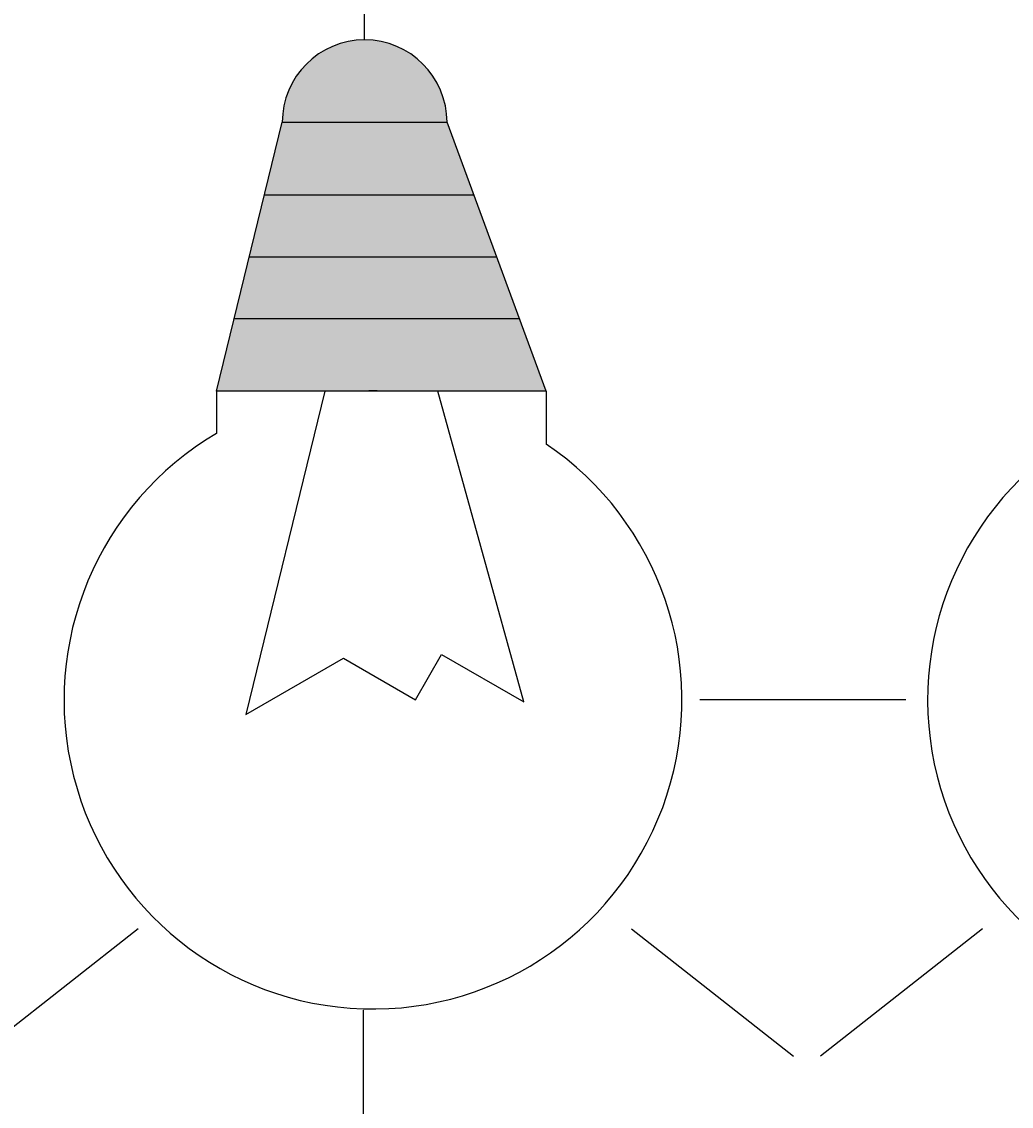
# Model space of a CAD drawing. Units: millimetres. Extents: x -8 to 285, y 5 to 221.
# Tile 26 of 30: x 172 to 221, y 132 to 185. Entities that reach past the tile are written whole.
import ezdxf

# ---------------------------------------------------------------- set-up
doc = ezdxf.new("R2010")
doc.units = ezdxf.units.MM
for name, color, linetype, lineweight in [('A-ANNO-DIMS', 2, 'Continuous', 18), ('E-EQPM-PATT', 252, 'Continuous', 13), ('E-LITE-FIXT', 7, 'Continuous', 25)]:
    doc.layers.add(name, color=color, linetype=linetype, lineweight=lineweight)
doc.layers.add('E-POWR-AC-LINE', color=30, linetype='Continuous', lineweight=25, true_color=0xf26722)
doc.styles.get("Standard").update_dxf_attribs({"font": 'arial.ttf'})
doc.dimstyles.get("Standard").update_dxf_attribs({"dimtxt": 0.18, "dimasz": 0.18, "dimexe": 0.18, "dimexo": 0.0625, "dimgap": 0.09, "dimtad": 0, "dimtih": 1, "dimtoh": 1, "dimdec": 4, "dimzin": 0, "dimdsep": 46, "dimtxsty": 'Standard', "dimcen": 0.09, "dimadec": 0, "dimazin": 0, "dimtfac": 1, "dimtdec": 4, "dimtofl": 0, "dimtmove": 0, "dimatfit": 3, "dimfxl": 1, "dimtolj": 1, "dimtzin": 0, "dimarcsym": 0})

# ---------------------------------------------------------------- blocks, each defined once
blk = doc.blocks.new('LAMP-INCANDESCENT')
for p, q in [((7.407, 29.994), (10.595, 43.039)), ((23.407, 29.994), (18.595, 43.039)), ((9.734, 39.517), (19.894, 39.517)), ((9.001, 36.517), (21.001, 36.517)), ((8.268, 33.517), (22.107, 33.517)), ((7.407, 29.994), (7.407, 27.935)), ((12.666, 29.994), (8.834, 14.293)), ((22.321, 14.903), (18.146, 29.994)), ((23.407, 29.994), (23.407, 27.423)), ((8.834, 14.293), (13.574, 17.029)), ((13.574, 17.029), (17.067, 15.012)), ((17.067, 15.012), (18.333, 17.205)), ((18.333, 17.205), (22.321, 14.903))]:
    blk.add_line(p, q)
for points in [[(10.595, 43.039), (18.595, 43.039)], [(23.407, 29.994), (7.407, 29.994)]]:
    blk.add_lwpolyline(points)
for centre, radius, start, end in [((14.595, 43.039), 4, 0, 180), ((15.001, 15), 15, 88.4488, 91.5512), ((15.001, 15), 15, 120.4152, 55.9163)]:
    blk.add_arc(centre, radius, start, end)
blk = doc.blocks.new('*D9')
at = {"layer": 'A-ANNO-DIMS', "color": 0, "lineweight": -2, "transparency": 16777216}
for p, q in [((6.672, 133.79), (6.672, 220.737)), ((270.919, 206.519), (270.919, 220.737)), ((6.852, 220.557), (138.33, 220.557)), ((270.739, 220.557), (139.262, 220.557))]:
    blk.add_line(p, q, dxfattribs=at)
at = {"layer": 'A-ANNO-DIMS', "color": 0, "transparency": 16777216}
for points in [[(6.852, 220.587), (6.852, 220.527), (6.672, 220.557)], [(270.739, 220.587), (270.739, 220.527), (270.919, 220.557)]]:
    blk.add_solid(points, dxfattribs=at)
at = {"layer": 'Defpoints', "color": 0, "transparency": 16777216}
for p in [(270.919, 220.557), (270.919, 206.457), (6.672, 133.727)]:
    blk.add_point(p, dxfattribs=at)
at = {"layer": 'A-ANNO-DIMS', "color": 0, "transparency": 16777216, "insert": (138.796, 220.557), "char_height": 0.18, "attachment_point": 5}
blk.add_mtext('\\A1;264.25', dxfattribs=at)
blk = doc.blocks.new('*D13')
at = {"layer": 'A-ANNO-DIMS', "color": 0, "lineweight": -2, "transparency": 16777216}
for p, q in [((145.21, 137.013), (145.21, 5.222)), ((189.039, 137.013), (189.039, 5.222)), ((145.39, 5.402), (166.727, 5.402)), ((188.859, 5.402), (167.522, 5.402))]:
    blk.add_line(p, q, dxfattribs=at)
at = {"layer": 'A-ANNO-DIMS', "color": 0, "transparency": 16777216}
for points in [[(145.39, 5.432), (145.39, 5.372), (145.21, 5.402)], [(188.859, 5.432), (188.859, 5.372), (189.039, 5.402)]]:
    blk.add_solid(points, dxfattribs=at)
at = {"layer": 'Defpoints', "color": 0, "transparency": 16777216}
for p in [(145.21, 137.075), (189.039, 137.075), (189.039, 5.402)]:
    blk.add_point(p, dxfattribs=at)
at = {"layer": 'A-ANNO-DIMS', "color": 0, "transparency": 16777216, "insert": (167.124, 5.402), "char_height": 0.18, "attachment_point": 5}
blk.add_mtext('\\A1;43.83', dxfattribs=at)
blk = doc.blocks.new('*D14')
at = {"layer": 'A-ANNO-DIMS', "color": 0, "lineweight": -2, "transparency": 16777216}
for p, q in [((189.039, 137.013), (189.039, 5.222)), ((230.967, 137.013), (230.967, 5.222)), ((189.219, 5.402), (209.606, 5.402)), ((230.787, 5.402), (210.4, 5.402))]:
    blk.add_line(p, q, dxfattribs=at)
at = {"layer": 'A-ANNO-DIMS', "color": 0, "transparency": 16777216}
for points in [[(189.219, 5.432), (189.219, 5.372), (189.039, 5.402)], [(230.787, 5.432), (230.787, 5.372), (230.967, 5.402)]]:
    blk.add_solid(points, dxfattribs=at)
at = {"layer": 'Defpoints', "color": 0, "transparency": 16777216}
for p in [(189.039, 137.075), (230.967, 137.075), (230.967, 5.402)]:
    blk.add_point(p, dxfattribs=at)
at = {"layer": 'A-ANNO-DIMS', "color": 0, "transparency": 16777216, "insert": (210.003, 5.402), "char_height": 0.18, "attachment_point": 5}
blk.add_mtext('\\A1;41.93', dxfattribs=at)

msp = doc.modelspace()

# ---------------------------------------------------------------- hatches: boundary and pattern name
at = {"layer": 'E-EQPM-PATT'}
h = msp.add_hatch(color=256, dxfattribs=at)
h.set_gradient(color1=(0, 0, 255), color2=(34, 52, 110), tint=1)
h.paths.add_polyline_path([(141.2836, 180.1071), (149.2836, 180.1071, 1)])
h.paths.add_polyline_path([(149.2836, 180.1071), (141.2836, 180.1071), (140.4228, 176.5846), (150.583, 176.5846)])
h.paths.add_polyline_path([(150.583, 176.5846), (140.4228, 176.5846), (139.6897, 173.5846), (151.6897, 173.5846)])
h.paths.add_polyline_path([(151.6897, 173.5846), (139.6897, 173.5846), (138.9565, 170.5846), (152.7963, 170.5846)])
h.paths.add_polyline_path([(152.7963, 170.5846), (138.9565, 170.5846), (138.0957, 167.062), (145.2836, 167.062, -0.0135377), (146.0957, 167.062), (154.0957, 167.062)])
h.paths.add_polyline_path([(193.1131, 180.1071), (185.1131, 180.1071), (184.2522, 176.5846), (194.4125, 176.5846)])
h.paths.add_polyline_path([(185.1131, 180.1071), (193.1131, 180.1071, 1)])
h.paths.add_polyline_path([(194.4125, 176.5846), (184.2522, 176.5846), (183.5191, 173.5846), (195.5191, 173.5846)])
h.paths.add_polyline_path([(195.5191, 173.5846), (183.5191, 173.5846), (182.786, 170.5846), (196.6258, 170.5846)])
h.paths.add_polyline_path([(196.6258, 170.5846), (182.786, 170.5846), (181.9252, 167.062), (189.1131, 167.062, -0.0135377), (189.9252, 167.062), (197.9252, 167.062)])
h.paths.add_polyline_path([(227.0413, 180.1071), (235.0413, 180.1071, 1)])
h.paths.add_polyline_path([(235.0413, 180.1071), (227.0413, 180.1071), (226.1804, 176.5846), (236.3407, 176.5846)])
h.paths.add_polyline_path([(236.3407, 176.5846), (226.1804, 176.5846), (225.4473, 173.5846), (237.4473, 173.5846)])
h.paths.add_polyline_path([(237.4473, 173.5846), (225.4473, 173.5846), (224.7142, 170.5846), (238.554, 170.5846)])
h.paths.add_polyline_path([(238.554, 170.5846), (224.7142, 170.5846), (223.8534, 167.062), (231.0413, 167.062, -0.0135377), (231.8534, 167.062), (239.8534, 167.062)])
h = msp.add_hatch(color=256, dxfattribs=at)
h.set_gradient(color2=(0, 0, 0), tint=1)
h.paths.add_polyline_path([(149.2836, 180.1071, 1), (141.2836, 180.1071)])
h.paths.add_polyline_path([(193.1131, 180.1071, 1), (185.1131, 180.1071)])
h.paths.add_polyline_path([(227.0413, 180.1071), (235.0413, 180.1071, 1)])

# ---------------------------------------------------------------- linework, layer by layer
at = {"layer": 'E-LITE-FIXT'}
for p, q in [((215.3855, 152.0675), (205.3855, 152.0675)), ((178.1125, 140.9643), (170.2549, 134.7789)), ((202.0747, 140.9643), (209.9322, 134.7789)), ((219.1045, 140.9643), (211.247, 134.7789))]:
    msp.add_line(p, q, dxfattribs=at)
at = {"layer": 'E-POWR-AC-LINE'}
msp.add_line((189.1131, 184.1071), (189.1131, 191.4908), dxfattribs=at)

# ---------------------------------------------------------------- block references
at = {"layer": 'E-LITE-FIXT'}
for p in [(174.5185, 137.068), (216.4466, 137.068)]:
    msp.add_blockref('LAMP-INCANDESCENT', p, dxfattribs=at)

# ---------------------------------------------------------------- dimensions: what is measured, and where the dimension line sits
at = {"layer": 'A-ANNO-DIMS'}
for base, p1, p2, picture, middle in [((270.9192, 220.5568), (6.6725, 133.7273), (270.9192, 206.4568), '*D9', (138.7958, 220.5568)), ((189.039, 5.402), (145.2095, 137.0752), (189.039, 137.0752), '*D13', (167.1243, 5.402)), ((230.9672, 5.402), (189.039, 137.0752), (230.9672, 137.0752), '*D14', (210.0031, 5.402))]:
    dim = msp.add_linear_dim(base=base, p1=p1, p2=p2, dimstyle='Standard', override={"dimdec": 2, "dimlfac": 1, "dimrnd": 0, "dimzin": 0, "dimdsep": 46, "dimlunit": 2}, dxfattribs=at)
    dim.commit()
    dim.dimension.update_dxf_attribs({"geometry": picture, "text_midpoint": middle})

doc.saveas('drawing.dxf')
